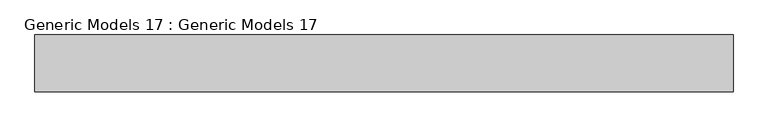
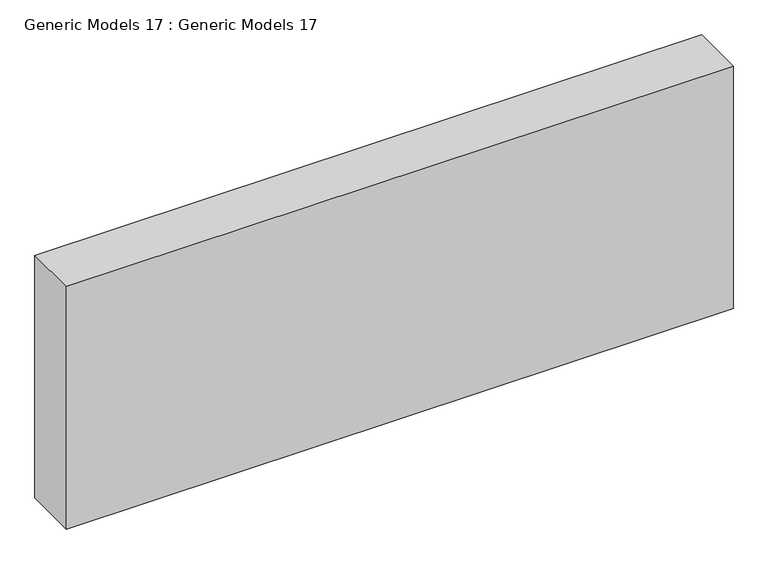
"""IFC4 building model written with IfcOpenShell, lengths in millimetres: proxy geometry, Generic Models 17 : Generic Models 17."""

from ifc_helpers import new_model, si_unit, origin, origin_with_axes, place, context, project, spatial, polyline, outline, extrude, source, transform, mapped, element, save


def generic_models_17_generic_models_17_a4f02c47(model_context):
    return source(origin(), model_context, "Body", "SweptSolid", [
        extrude(outline(polyline([(4014.2938154, -7687.0227991), (4014.2938154, -8039.7013811), (-311.2292634, -8039.7013811), (-311.2292634, -7687.0227991), (4014.2938154, -7687.0227991)])), origin_with_axes(), (0.0, 0.0, 1.0), 1664.0724017),
    ])


if __name__ == "__main__":
    model = new_model("IFC4")
    model_context = context("Model", 3, world=origin())
    ifc_project = project(units=[si_unit("LENGTHUNIT", "METRE", prefix="MILLI")], contexts=[model_context])
    site = spatial("IfcSite", under=ifc_project)
    building = spatial("IfcBuilding", under=site)
    placement = place(None, origin())
    generic_models_17_generic_models_17_shape = generic_models_17_generic_models_17_a4f02c47(model_context)
    element("IfcBuildingElementProxy", 1, Name="Generic Models 17 : Generic Models 17", ObjectType="Generic Models 17 : Generic Models 17", at=placement, inside=building, context=model_context, shape_type="MappedRepresentation", body=[
        mapped(generic_models_17_generic_models_17_shape, transform((0.0, 0.0, 0.0), x_axis=(1.0, 0.0, 0.0), y_axis=(0.0, 1.0, 0.0), z_axis=(0.0, 0.0, 1.0))),
    ])
    save(model, "model.ifc")
